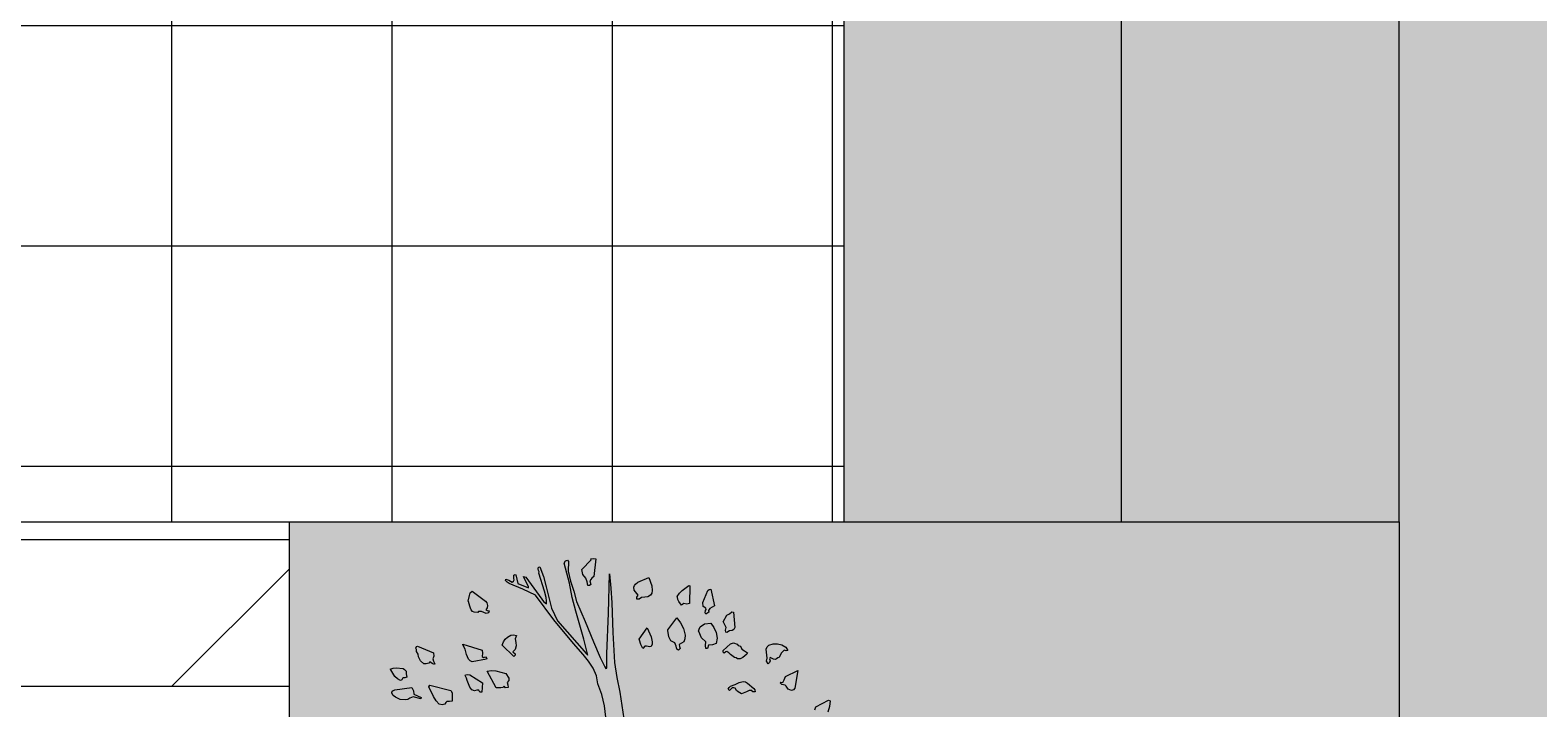
# Model space of a CAD drawing. Units: inches. Extents: x 84 to 1044, y -280 to 906.
# Tile 63 of 105: x 375 to 440, y 761 to 790. Entities that reach past the tile are written whole.
import ezdxf

# ---------------------------------------------------------------- set-up
doc = ezdxf.new("R2010")
doc.units = ezdxf.units.IN
for name, color, linetype, lineweight in [('A-ANNO-DIMS', 2, 'Continuous', 18), ('A-STAIRCASE', 144, 'Continuous', 18), ('L-HRDS', 32, 'Continuous', 18), ('L-PLNT', 114, 'Continuous', 15)]:
    doc.layers.add(name, color=color, linetype=linetype, lineweight=lineweight)
for name, color, linetype, lineweight, true_color in [('A-FLOR-PATT', 251, 'Continuous', 9, 0x705861), ('A-FLOR-STRS-PATT', 35, 'Continuous', 9, 0x947764), ('L-PLNT-PATT', 9, 'Continuous', 9, 0xafd9aa)]:
    doc.layers.add(name, color=color, linetype=linetype, lineweight=lineweight, true_color=true_color)
doc.styles.get("Standard").update_dxf_attribs({"font": 'arial.ttf'})
doc.dimstyles.get("Standard").update_dxf_attribs({"dimtxt": 0.18, "dimasz": 0.18, "dimexe": 0.18, "dimexo": 0.0625, "dimgap": 0.09, "dimtad": 0, "dimtih": 1, "dimtoh": 1, "dimdec": 4, "dimzin": 0, "dimdsep": 46, "dimtxsty": 'Standard', "dimcen": 0.09, "dimadec": 0, "dimazin": 0, "dimtfac": 1, "dimtdec": 4, "dimtofl": 0, "dimtmove": 0, "dimatfit": 3, "dimfxl": 1, "dimtolj": 1, "dimtzin": 0, "dimarcsym": 0})

# ---------------------------------------------------------------- blocks, each defined once
blk = doc.blocks.new('A$C37E508DF')
for p, q in [((0.6329, 1.5111), (0.6367, 1.5175)), ((0.6475, 1.4545), (0.6329, 1.5111)), ((0.6367, 1.5175), (0.6423, 1.5201)), ((0.6423, 1.5201), (0.6453, 1.5158)), ((0.6453, 1.5158), (0.644, 1.4879)), ((0.6826, 1.493), (0.7096, 1.5209)), ((0.7083, 1.5239), (0.7152, 1.5244)), ((0.7096, 1.5209), (0.7083, 1.5239)), ((0.7152, 1.5244), (0.7225, 1.5231)), ((0.7225, 1.5231), (0.7174, 1.4729)), ((0.4657, 1.4622), (0.4669, 1.4652)), ((0.4708, 1.4566), (0.4657, 1.4622)), ((0.4669, 1.4652), (0.4755, 1.463)), ((0.4755, 1.463), (0.4845, 1.4575)), ((0.4845, 1.4575), (0.4884, 1.4596)), ((0.4884, 1.4596), (0.4905, 1.4635)), ((0.4897, 1.4772), (0.4935, 1.4789)), ((0.4897, 1.4678), (0.4897, 1.4772)), ((0.4905, 1.4635), (0.4897, 1.4678)), ((0.4935, 1.4789), (0.4952, 1.478)), ((0.4952, 1.478), (0.5004, 1.4532)), ((0.5313, 1.4437), (0.5167, 1.4729)), ((0.5167, 1.4729), (0.5231, 1.4716)), ((0.5231, 1.4716), (0.5686, 1.409)), ((0.5583, 1.4948), (0.5596, 1.4995)), ((0.5596, 1.4905), (0.5583, 1.4948)), ((0.5596, 1.4995), (0.563, 1.5003)), ((0.5613, 1.4862), (0.5596, 1.4905)), ((0.5608, 1.4823), (0.5613, 1.4862)), ((0.5767, 1.4317), (0.5608, 1.4823)), ((0.563, 1.5003), (0.5737, 1.4733)), ((0.5737, 1.4733), (0.5814, 1.4437)), ((0.644, 1.4879), (0.6505, 1.46)), ((0.6505, 1.46), (0.6603, 1.4317)), ((0.6852, 1.4785), (0.6826, 1.493)), ((0.6946, 1.4682), (0.6852, 1.4785)), ((0.6976, 1.4579), (0.6946, 1.4682)), ((0.7109, 1.4682), (0.7053, 1.4609)), ((0.7053, 1.4609), (0.7083, 1.4502)), ((0.7174, 1.4729), (0.7109, 1.4682)), ((0.7589, 1.3691), (0.7615, 1.481)), ((0.7615, 1.481), (0.7658, 1.4395)), ((0.8421, 1.4575), (0.8739, 1.4703)), ((0.8739, 1.4703), (0.882, 1.4463)), ((0.3598, 1.403), (0.3628, 1.4189)), ((0.3628, 1.4189), (0.3649, 1.4266)), ((0.3649, 1.4266), (0.3709, 1.4317)), ((0.3709, 1.4317), (0.4086, 1.403)), ((0.4764, 1.4532), (0.4708, 1.4566)), ((0.5154, 1.4373), (0.4764, 1.4532)), ((0.5004, 1.4532), (0.5308, 1.4412)), ((0.551, 1.4197), (0.5154, 1.4373)), ((0.5308, 1.4412), (0.5313, 1.4437)), ((0.6029, 1.3494), (0.551, 1.4197)), ((0.5814, 1.4133), (0.5767, 1.4317)), ((0.5814, 1.4437), (0.5969, 1.3833)), ((0.6552, 1.4137), (0.6475, 1.4545)), ((0.6603, 1.4317), (0.668, 1.4021)), ((0.7002, 1.4476), (0.6976, 1.4579)), ((0.7049, 1.448), (0.7002, 1.4476)), ((0.7083, 1.4502), (0.7049, 1.448)), ((0.7658, 1.4395), (0.7684, 1.3979)), ((0.831, 1.4424), (0.8323, 1.4476)), ((0.8318, 1.4343), (0.831, 1.4424)), ((0.8353, 1.4292), (0.8318, 1.4343)), ((0.8323, 1.4476), (0.8357, 1.451)), ((0.8434, 1.4197), (0.8353, 1.4292)), ((0.8357, 1.451), (0.8421, 1.4575)), ((0.8391, 1.4141), (0.8434, 1.4197)), ((0.8781, 1.4197), (0.8709, 1.4154)), ((0.8816, 1.4262), (0.8781, 1.4197)), ((0.8829, 1.433), (0.8816, 1.4262)), ((0.882, 1.4463), (0.8829, 1.433)), ((0.9545, 1.4159), (0.9605, 1.4257)), ((0.9549, 1.4146), (0.9545, 1.4159)), ((0.9605, 1.4257), (0.9686, 1.4334)), ((0.9686, 1.4334), (0.9875, 1.4476)), ((0.9875, 1.4476), (0.9905, 1.4467)), ((0.9905, 1.4467), (0.9896, 1.3966)), ((1.0269, 1.3996), (1.0411, 1.433)), ((1.0411, 1.433), (1.045, 1.4365)), ((1.045, 1.4365), (1.0497, 1.4369)), ((1.0497, 1.4369), (1.0604, 1.3901)), ((0.3602, 1.4021), (0.3598, 1.403)), ((0.364, 1.3888), (0.3602, 1.4021)), ((0.3657, 1.3828), (0.364, 1.3888)), ((0.3683, 1.3781), (0.3657, 1.3828)), ((0.3718, 1.3738), (0.3683, 1.3781)), ((0.3765, 1.3713), (0.3718, 1.3738)), ((0.3885, 1.3738), (0.3872, 1.3708)), ((0.3971, 1.3734), (0.3885, 1.3738)), ((0.4039, 1.3704), (0.3971, 1.3734)), ((0.4086, 1.403), (0.4125, 1.3979)), ((0.4134, 1.3837), (0.4099, 1.3781)), ((0.4099, 1.3781), (0.4134, 1.376)), ((0.4125, 1.3979), (0.4142, 1.391)), ((0.4142, 1.391), (0.4134, 1.3837)), ((0.4134, 1.376), (0.4189, 1.3751)), ((0.4189, 1.3751), (0.4176, 1.37)), ((0.5686, 1.409), (0.5741, 1.4021)), ((0.5741, 1.4021), (0.5823, 1.3953)), ((0.5827, 1.4043), (0.5814, 1.4133)), ((0.5823, 1.3953), (0.5827, 1.4043)), ((0.5969, 1.3833), (0.6132, 1.3472)), ((0.6655, 1.3743), (0.6552, 1.4137)), ((0.6882, 1.2949), (0.6655, 1.3743)), ((0.668, 1.4021), (0.6925, 1.3455)), ((0.7684, 1.3979), (0.771, 1.3134)), ((0.8395, 1.4086), (0.8391, 1.4141)), ((0.846, 1.4086), (0.8395, 1.4086)), ((0.8528, 1.4137), (0.846, 1.4086)), ((0.8619, 1.4146), (0.8528, 1.4137)), ((0.8709, 1.4154), (0.8619, 1.4146)), ((0.9558, 1.4077), (0.9549, 1.4146)), ((0.9592, 1.4017), (0.9558, 1.4077)), ((0.966, 1.3914), (0.9592, 1.4017)), ((0.9703, 1.3944), (0.966, 1.3914)), ((0.9733, 1.3966), (0.9703, 1.3944)), ((0.9819, 1.3944), (0.9733, 1.3966)), ((0.9896, 1.3966), (0.9819, 1.3944)), ((1.0282, 1.3876), (1.0269, 1.3996)), ((1.0359, 1.3833), (1.0282, 1.3876)), ((1.0334, 1.37), (1.0351, 1.376)), ((1.0351, 1.376), (1.0368, 1.3794)), ((1.0368, 1.3794), (1.0359, 1.3833)), ((1.0471, 1.3824), (1.0432, 1.3764)), ((1.0432, 1.3764), (1.0441, 1.3717)), ((1.0604, 1.3901), (1.0471, 1.3824)), ((1.1033, 1.367), (1.1097, 1.373)), ((1.1097, 1.373), (1.114, 1.3717)), ((0.3872, 1.3708), (0.3765, 1.3713)), ((0.4108, 1.3683), (0.4039, 1.3704)), ((0.4176, 1.37), (0.4108, 1.3683)), ((0.6595, 1.2829), (0.6029, 1.3494)), ((0.6132, 1.3472), (0.6959, 1.2529)), ((0.6925, 1.3455), (0.7161, 1.2868)), ((0.7538, 1.2529), (0.7589, 1.3691)), ((0.9274, 1.3215), (0.9532, 1.3554)), ((0.9532, 1.3554), (0.9635, 1.3413)), ((0.9635, 1.3413), (0.9721, 1.325)), ((1.0197, 1.3297), (1.0321, 1.3387)), ((1.0321, 1.3387), (1.0497, 1.3404)), ((1.0359, 1.3661), (1.0334, 1.37)), ((1.0441, 1.3717), (1.0359, 1.3661)), ((1.0497, 1.3404), (1.0587, 1.3284)), ((1.0848, 1.3443), (1.0955, 1.3631)), ((1.0861, 1.343), (1.0848, 1.3443)), ((1.0938, 1.328), (1.0861, 1.343)), ((1.0955, 1.3631), (1.1033, 1.367)), ((1.114, 1.3717), (1.1183, 1.328)), ((0.4597, 1.2868), (0.4648, 1.2945)), ((0.4648, 1.2945), (0.4717, 1.3009)), ((0.4717, 1.3009), (0.4807, 1.3065)), ((0.4807, 1.3065), (0.4884, 1.3074)), ((0.4884, 1.3074), (0.4965, 1.3057)), ((0.4965, 1.3057), (0.4935, 1.2954)), ((0.4935, 1.2954), (0.4948, 1.2855)), ((0.7002, 1.2495), (0.6882, 1.2949)), ((0.771, 1.3134), (0.7761, 1.2285)), ((0.846, 1.2949), (0.8687, 1.3271)), ((0.8473, 1.2924), (0.846, 1.2949)), ((0.8507, 1.2795), (0.8473, 1.2924)), ((0.8687, 1.3271), (0.8803, 1.3014)), ((0.8803, 1.3014), (0.8833, 1.2872)), ((0.8833, 1.2872), (0.8829, 1.2808)), ((0.9279, 1.3194), (0.9274, 1.3215)), ((0.9305, 1.3018), (0.9279, 1.3194)), ((0.9365, 1.2902), (0.9305, 1.3018)), ((0.9476, 1.2842), (0.9365, 1.2902)), ((0.9721, 1.325), (0.9768, 1.3061)), ((0.9763, 1.2962), (0.9733, 1.2868)), ((0.9768, 1.3061), (0.9763, 1.2962)), ((1.0149, 1.3172), (1.0171, 1.3232)), ((1.0162, 1.3164), (1.0149, 1.3172)), ((1.0231, 1.2988), (1.0162, 1.3164)), ((1.0171, 1.3232), (1.0197, 1.3297)), ((1.0359, 1.2868), (1.0231, 1.2988)), ((1.0587, 1.3284), (1.0651, 1.3134)), ((1.0677, 1.2975), (1.0647, 1.2829)), ((1.0651, 1.3134), (1.0677, 1.2975)), ((1.0917, 1.3207), (1.0938, 1.328)), ((1.0925, 1.3151), (1.0917, 1.3207)), ((1.0955, 1.3138), (1.0925, 1.3151)), ((1.1028, 1.3185), (1.0955, 1.3138)), ((1.111, 1.3194), (1.1028, 1.3185)), ((1.1153, 1.3228), (1.111, 1.3194)), ((1.1183, 1.328), (1.1153, 1.3228)), ((0.2101, 1.2696), (0.2127, 1.2744)), ((0.2127, 1.2654), (0.2101, 1.2696)), ((0.2127, 1.2744), (0.2152, 1.2752)), ((0.2127, 1.2602), (0.2127, 1.2654)), ((0.2174, 1.2521), (0.2127, 1.2602)), ((0.2152, 1.2752), (0.2611, 1.2559)), ((0.2182, 1.2443), (0.2174, 1.2521)), ((0.2234, 1.2336), (0.2182, 1.2443)), ((0.262, 1.2465), (0.2586, 1.2388)), ((0.2611, 1.2559), (0.262, 1.2465)), ((0.3439, 1.2804), (0.3992, 1.2636)), ((0.3439, 1.2787), (0.3439, 1.2804)), ((0.3507, 1.2662), (0.3439, 1.2787)), ((0.3546, 1.2516), (0.3507, 1.2662)), ((0.3602, 1.2383), (0.3546, 1.2516)), ((0.3992, 1.2636), (0.4005, 1.2546)), ((0.4005, 1.2546), (0.3992, 1.2452)), ((0.3992, 1.2452), (0.4026, 1.2431)), ((0.4026, 1.2431), (0.4086, 1.2443)), ((0.4086, 1.2443), (0.4121, 1.2401)), ((0.4562, 1.2774), (0.4597, 1.2868)), ((0.4897, 1.2452), (0.4562, 1.2774)), ((0.4935, 1.2658), (0.4867, 1.2589)), ((0.4867, 1.2589), (0.4935, 1.2529)), ((0.4931, 1.2491), (0.4897, 1.2452)), ((0.4935, 1.2529), (0.4931, 1.2491)), ((0.4961, 1.2756), (0.4935, 1.2658)), ((0.4948, 1.2855), (0.4961, 1.2756)), ((0.6865, 1.2508), (0.6595, 1.2829)), ((0.7015, 1.2323), (0.6865, 1.2508)), ((0.6959, 1.2529), (0.7002, 1.2495)), ((0.7161, 1.2868), (0.7349, 1.2422)), ((0.7538, 1.2122), (0.7538, 1.2529)), ((0.8567, 1.2679), (0.8507, 1.2795)), ((0.8619, 1.2752), (0.8567, 1.2679)), ((0.867, 1.2752), (0.8619, 1.2752)), ((0.8713, 1.2739), (0.867, 1.2752)), ((0.8756, 1.2726), (0.8713, 1.2739)), ((0.8799, 1.2744), (0.8756, 1.2726)), ((0.8829, 1.2808), (0.8799, 1.2744)), ((0.951, 1.2748), (0.9476, 1.2842)), ((0.9532, 1.2666), (0.951, 1.2748)), ((0.9583, 1.2636), (0.9532, 1.2666)), ((0.9626, 1.2679), (0.9583, 1.2636)), ((0.9733, 1.2868), (0.9596, 1.2799)), ((0.9596, 1.2799), (0.9605, 1.2744)), ((0.9605, 1.2744), (0.9626, 1.2679)), ((1.0347, 1.2769), (1.0359, 1.2868)), ((1.0359, 1.2679), (1.0347, 1.2769)), ((1.0402, 1.2679), (1.0359, 1.2679)), ((1.0432, 1.2774), (1.0402, 1.2679)), ((1.0544, 1.2791), (1.0432, 1.2774)), ((1.0647, 1.2829), (1.0544, 1.2791)), ((1.0848, 1.2628), (1.1054, 1.2817)), ((1.0852, 1.2576), (1.0848, 1.2628)), ((1.0883, 1.2546), (1.0852, 1.2576)), ((1.0921, 1.2585), (1.0883, 1.2546)), ((1.0955, 1.2602), (1.0921, 1.2585)), ((1.1015, 1.2559), (1.0955, 1.2602)), ((1.1063, 1.2508), (1.1015, 1.2559)), ((1.1054, 1.2817), (1.1148, 1.2842)), ((1.117, 1.2422), (1.1063, 1.2508)), ((1.1148, 1.2842), (1.1247, 1.2804)), ((1.1247, 1.2804), (1.1281, 1.2765)), ((1.1281, 1.2765), (1.1341, 1.2752)), ((1.1341, 1.2752), (1.1384, 1.2666)), ((1.1384, 1.2666), (1.1461, 1.2619)), ((1.1526, 1.2521), (1.141, 1.2422)), ((1.1461, 1.2619), (1.1539, 1.2559)), ((1.1539, 1.2559), (1.1526, 1.2521)), ((1.2075, 1.2666), (1.21, 1.2726)), ((1.2096, 1.2491), (1.2075, 1.2666)), ((1.21, 1.2409), (1.2096, 1.2491)), ((1.21, 1.2726), (1.2147, 1.2774)), ((1.2147, 1.2774), (1.2276, 1.2817)), ((1.2276, 1.2817), (1.2392, 1.2817)), ((1.2392, 1.2817), (1.2521, 1.2787)), ((1.2503, 1.2551), (1.2448, 1.2431)), ((1.2585, 1.2636), (1.2503, 1.2551)), ((1.2521, 1.2787), (1.2632, 1.2722)), ((1.2645, 1.2615), (1.2585, 1.2636)), ((1.2632, 1.2722), (1.2692, 1.2628)), ((1.2692, 1.2628), (1.2645, 1.2615)), ((0.1376, 1.2092), (0.1458, 1.2126)), ((0.1389, 1.2079), (0.1376, 1.2092)), ((0.1505, 1.189), (0.1389, 1.2079)), ((0.1458, 1.2126), (0.1548, 1.2135)), ((0.1548, 1.2135), (0.1741, 1.2109)), ((0.1741, 1.2109), (0.1784, 1.2083)), ((0.1784, 1.2083), (0.1831, 1.204)), ((0.1831, 1.204), (0.1831, 1.1959)), ((0.2328, 1.2251), (0.2234, 1.2336)), ((0.2401, 1.2251), (0.2328, 1.2251)), ((0.2474, 1.2268), (0.2401, 1.2251)), ((0.2504, 1.2306), (0.2474, 1.2268)), ((0.2568, 1.2255), (0.2504, 1.2306)), ((0.2633, 1.2229), (0.2568, 1.2255)), ((0.2586, 1.2388), (0.2611, 1.2319)), ((0.2611, 1.2319), (0.265, 1.2251)), ((0.265, 1.2251), (0.2633, 1.2229)), ((0.3649, 1.2336), (0.3602, 1.2383)), ((0.3709, 1.2306), (0.3649, 1.2336)), ((0.4112, 1.2375), (0.3709, 1.2306)), ((0.4121, 1.2401), (0.4112, 1.2375)), ((0.4134, 1.204), (0.4258, 1.2058)), ((0.4391, 1.156), (0.4134, 1.204)), ((0.4258, 1.2058), (0.4382, 1.2045)), ((0.4382, 1.2045), (0.4669, 1.1972)), ((0.7148, 1.2126), (0.7015, 1.2323)), ((0.7246, 1.1908), (0.7148, 1.2126)), ((0.7349, 1.2422), (0.7482, 1.216)), ((0.7482, 1.216), (0.7508, 1.2109)), ((0.7508, 1.2109), (0.7538, 1.2122)), ((0.7761, 1.2285), (0.7821, 1.1856)), ((1.1221, 1.2418), (1.117, 1.2422)), ((1.126, 1.2388), (1.1221, 1.2418)), ((1.1337, 1.2388), (1.126, 1.2388)), ((1.141, 1.2422), (1.1337, 1.2388)), ((1.2079, 1.2323), (1.21, 1.2409)), ((1.2126, 1.2251), (1.2079, 1.2323)), ((1.2169, 1.2285), (1.2126, 1.2251)), ((1.2186, 1.2332), (1.2169, 1.2285)), ((1.2186, 1.2431), (1.2173, 1.2392)), ((1.2173, 1.2392), (1.2186, 1.2332)), ((1.2285, 1.2383), (1.2186, 1.2431)), ((1.2328, 1.2366), (1.2285, 1.2383)), ((1.2371, 1.2388), (1.2328, 1.2366)), ((1.2405, 1.2418), (1.2371, 1.2388)), ((1.2448, 1.2431), (1.2405, 1.2418)), ((1.2628, 1.1882), (1.2975, 1.2053)), ((1.2975, 1.2053), (1.2885, 1.1556)), ((0.1582, 1.1822), (0.1505, 1.189)), ((0.1668, 1.1775), (0.1582, 1.1822)), ((0.1711, 1.1792), (0.1668, 1.1775)), ((0.1728, 1.1826), (0.1711, 1.1792)), ((0.1758, 1.1847), (0.1728, 1.1826)), ((0.1788, 1.1852), (0.1758, 1.1847)), ((0.1848, 1.1865), (0.1788, 1.1852)), ((0.1831, 1.1959), (0.1848, 1.1865)), ((0.2478, 1.1594), (0.2504, 1.1637)), ((0.2607, 1.1316), (0.2478, 1.1594)), ((0.2504, 1.1637), (0.3104, 1.1487)), ((0.3507, 1.1916), (0.352, 1.1933)), ((0.355, 1.1839), (0.3507, 1.1916)), ((0.352, 1.1933), (0.3576, 1.1942)), ((0.3563, 1.177), (0.355, 1.1839)), ((0.3645, 1.1586), (0.3563, 1.177)), ((0.3576, 1.1942), (0.364, 1.1929)), ((0.364, 1.1929), (0.4005, 1.1702)), ((0.37, 1.1509), (0.3645, 1.1586)), ((0.4005, 1.1702), (0.3979, 1.1436)), ((0.4622, 1.1607), (0.458, 1.1573)), ((0.4657, 1.156), (0.4622, 1.1607)), ((0.4669, 1.1972), (0.4747, 1.1843)), ((0.4751, 1.177), (0.47, 1.1714)), ((0.47, 1.1714), (0.4721, 1.1646)), ((0.4721, 1.1646), (0.473, 1.1573)), ((0.4747, 1.1843), (0.4751, 1.177)), ((0.7281, 1.168), (0.7246, 1.1908)), ((0.7396, 1.1371), (0.7281, 1.168)), ((0.7821, 1.1856), (0.7911, 1.1436)), ((1.102, 1.1573), (1.1063, 1.1612)), ((1.1063, 1.1612), (1.1187, 1.1655)), ((1.1187, 1.1655), (1.1307, 1.1714)), ((1.1307, 1.1714), (1.1423, 1.1744)), ((1.1423, 1.1744), (1.1483, 1.1732)), ((1.1483, 1.1732), (1.1539, 1.1693)), ((1.1539, 1.1693), (1.1727, 1.1543)), ((1.2469, 1.1702), (1.2495, 1.1723)), ((1.2478, 1.1693), (1.2469, 1.1702)), ((1.2516, 1.1659), (1.2478, 1.1693)), ((1.2495, 1.1723), (1.2546, 1.1719)), ((1.2563, 1.1646), (1.2516, 1.1659)), ((1.2546, 1.1719), (1.2589, 1.1792)), ((1.2611, 1.1637), (1.2563, 1.1646)), ((1.2589, 1.1792), (1.2628, 1.1882)), ((1.2641, 1.1612), (1.2611, 1.1637)), ((1.2701, 1.1522), (1.2641, 1.1612)), ((0.1419, 1.1436), (0.1449, 1.1474)), ((0.1419, 1.141), (0.1419, 1.1436)), ((0.1462, 1.1342), (0.1419, 1.141)), ((0.1449, 1.1474), (0.1509, 1.1504)), ((0.1522, 1.1294), (0.1462, 1.1342)), ((0.1509, 1.1504), (0.1994, 1.1573)), ((0.1655, 1.1234), (0.1522, 1.1294)), ((0.181, 1.1226), (0.1655, 1.1234)), ((0.1878, 1.1234), (0.181, 1.1226)), ((0.1938, 1.1273), (0.1878, 1.1234)), ((0.2032, 1.1303), (0.1938, 1.1273)), ((0.1994, 1.1573), (0.2041, 1.1479)), ((0.2247, 1.1251), (0.2032, 1.1303)), ((0.2041, 1.1479), (0.2045, 1.138)), ((0.2045, 1.138), (0.226, 1.129)), ((0.226, 1.129), (0.2247, 1.1251)), ((0.268, 1.1196), (0.2607, 1.1316)), ((0.277, 1.1101), (0.268, 1.1196)), ((0.2984, 1.1179), (0.2959, 1.1144)), ((0.3066, 1.1179), (0.2984, 1.1179)), ((0.3134, 1.1183), (0.3066, 1.1179)), ((0.3104, 1.1487), (0.3134, 1.1423)), ((0.3134, 1.1423), (0.3139, 1.1346)), ((0.3139, 1.1346), (0.3134, 1.1183)), ((0.3778, 1.1474), (0.37, 1.1509)), ((0.3842, 1.15), (0.3778, 1.1474)), ((0.3898, 1.15), (0.3842, 1.15)), ((0.3923, 1.1436), (0.3898, 1.15)), ((0.3979, 1.1436), (0.3923, 1.1436)), ((0.4519, 1.1564), (0.4391, 1.156)), ((0.458, 1.1573), (0.4519, 1.1564)), ((0.473, 1.1573), (0.4657, 1.156)), ((0.7469, 1.1054), (0.7396, 1.1371)), ((0.7911, 1.1436), (0.8027, 1.0677)), ((1.099, 1.153), (1.102, 1.1573)), ((1.1033, 1.1487), (1.099, 1.153)), ((1.111, 1.156), (1.1033, 1.1487)), ((1.1153, 1.1564), (1.111, 1.156)), ((1.1191, 1.1556), (1.1153, 1.1564)), ((1.1226, 1.1492), (1.1191, 1.1556)), ((1.1273, 1.1453), (1.1226, 1.1492)), ((1.1367, 1.1393), (1.1273, 1.1453)), ((1.1517, 1.1453), (1.1367, 1.1393)), ((1.1586, 1.1483), (1.1517, 1.1453)), ((1.1663, 1.1487), (1.1586, 1.1483)), ((1.1697, 1.1449), (1.1663, 1.1487)), ((1.1757, 1.1449), (1.1697, 1.1449)), ((1.1727, 1.1543), (1.1749, 1.1504)), ((1.1749, 1.1504), (1.1757, 1.1449)), ((1.2791, 1.1487), (1.2701, 1.1522)), ((1.2851, 1.1509), (1.2791, 1.1487)), ((1.2885, 1.1556), (1.2851, 1.1509)), ((1.3485, 1.102), (1.385, 1.1209)), ((1.385, 1.1209), (1.3897, 1.1196)), ((1.3897, 1.1196), (1.3875, 1.1037)), ((0.2856, 1.108), (0.277, 1.1101)), ((0.2933, 1.1101), (0.2856, 1.108)), ((0.2959, 1.1144), (0.2933, 1.1101)), ((0.7512, 1.0728), (0.7469, 1.1054)), ((1.3455, 1.0934), (1.3485, 1.102)), ((1.3875, 1.1037), (1.3828, 1.087))]:
    blk.add_line(p, q)
blk = doc.blocks.new('*D62')
at = {"layer": 'A-ANNO-DIMS', "color": 0, "lineweight": -2, "transparency": 16777216}
for p, q in [((203.179, 709.183), (203.179, 905.9)), ((203.359, 905.72), (549.232, 905.72)), ((895.894, 905.72), (550.021, 905.72)), ((896.074, 400.183), (896.074, 905.9))]:
    blk.add_line(p, q, dxfattribs=at)
at = {"layer": 'A-ANNO-DIMS', "color": 0, "transparency": 16777216}
for points in [[(203.359, 905.75), (203.359, 905.69), (203.179, 905.72)], [(895.894, 905.75), (895.894, 905.69), (896.074, 905.72)]]:
    blk.add_solid(points, dxfattribs=at)
at = {"layer": 'Defpoints', "color": 0, "transparency": 16777216}
for p in [(896.074, 905.72), (203.179, 709.12), (896.074, 400.12)]:
    blk.add_point(p, dxfattribs=at)
at = {"layer": 'A-ANNO-DIMS', "color": 0, "transparency": 16777216, "insert": (549.627, 905.72), "char_height": 0.18, "attachment_point": 5}
blk.add_mtext('\\A1;692.9', dxfattribs=at)

msp = doc.modelspace()

# ---------------------------------------------------------------- hatches: boundary and pattern name
at = {"layer": 'A-FLOR-PATT', "transparency": 33554597}
h = msp.add_hatch(dxfattribs=at)
h.set_pattern_fill('ANSI37', color=256, scale=3, angle=45)
h.paths.add_polyline_path([(410.074, 847.12), (143.179, 847.12), (143.179, 769.12), (203.179, 769.12), (410.074, 769.12)])
h.paths.add_polyline_path([(254.313, 826.374, -0.414214), (254.257, 823.878, -0.414214), (251.76, 823.934), (244.439, 831.592, 0.3775), (230.555, 830.526, 0.076599), (228.51, 828.052, -0.127919), (230.803, 827.709, -0.121523), (233.469, 828.328, -0.425989), (233.291, 814.163, -0.165541), (230.889, 815.094, -0.016888), (230.578, 814.914), (236.189, 809.046, -0.414214), (236.133, 806.549, -0.414214), (233.636, 806.605, 0.414214), (238.63, 806.493), (246.415, 813.937), (254.201, 821.381, 0.414214)], flags=16)
h.paths.add_polyline_path([(241.241, 801.211), (258.998, 817.357), (267.168, 808.372), (249.545, 792.347)], flags=16)
h.paths.add_polyline_path([(262.121, 832.717, -1), (274.121, 832.717, -1)], flags=16)
h.paths.add_polyline_path([(315.269, 832.717, -1), (327.269, 832.717, -1)], flags=16)
h.paths.add_polyline_path([(322.221, 808.372), (330.392, 817.357), (348.148, 801.211), (339.844, 792.347)], flags=16)
h.paths.add_polyline_path([(344.951, 831.592, -0.372719), (358.711, 830.652), (358.966, 830.408, -0.072384), (360.879, 828.052, -0.103042), (362.667, 827.476, -0.02342), (363.022, 827.039, 0.134832), (360.058, 831.805, 0.419104)], flags=0)
h.paths.add_polyline_path([(355.753, 806.605, -0.414214), (353.257, 806.549, -0.414214), (353.201, 809.046), (358.811, 814.914, 0.234158), (363.536, 814.769, 0.403722), (362.499, 834.358, 0.41788), (342.398, 834.032), (335.076, 826.374, 0.414214), (335.188, 821.381), (342.974, 813.937), (350.76, 806.493, 0.414214)], flags=16)
h = msp.add_hatch(dxfattribs=at)
h.set_pattern_fill('DOLMIT', color=256)
h.paths.add_polyline_path([(896.074, 709.12), (833.074, 709.12), (833.074, 646.12), (833.074, 574.12), (833.074, 511.12), (896.074, 511.12)])
h.paths.add_polyline_path([(386.074, 769.12), (203.179, 769.12), (203.179, 709.12), (287.127, 709.12), (359.127, 709.12), (386.074, 709.12)])
at = {"layer": 'A-FLOR-STRS-PATT', "transparency": 33554567}
h = msp.add_hatch(color=256, dxfattribs=at)
h.dxf.hatch_style = 1
h.paths.add_polyline_path([(650.074, 91.12), (638.074, 91.12), (638.074, 67.12), (455.074, 67.12), (455.074, 55.12), (650.074, 55.12)], flags=17)
h.paths.add_polyline_path([(662.074, 91.12), (650.074, 91.12), (650.074, 55.12), (455.074, 55.12), (455.074, 43.12), (662.074, 43.12)])
h.paths.add_polyline_path([(674.074, 91.12), (671.074, 91.12), (662.074, 91.12), (662.074, 43.12), (455.074, 43.12), (455.074, 31.12), (674.074, 31.12)])
h.paths.add_polyline_path([(227.179, 151.12), (203.179, 151.12), (143.179, 151.12), (143.179, 139.12), (227.179, 139.12)])
h.paths.add_polyline_path([(227.179, 139.12), (143.179, 139.12), (143.179, 127.12), (227.179, 127.12)])
h.paths.add_polyline_path([(203.179, 271.12), (143.179, 271.12), (143.179, 259.12), (203.179, 259.12)])
h.paths.add_polyline_path([(203.179, 259.12), (143.179, 259.12), (143.179, 247.12), (203.179, 247.12)])
h.paths.add_polyline_path([(203.179, 769.12), (143.179, 769.12), (143.179, 757.12), (203.179, 757.12)])
h.paths.add_polyline_path([(203.179, 757.12), (143.179, 757.12), (143.179, 745.12), (203.179, 745.12)])
h.paths.add_polyline_path([(434.074, 847.12), (422.074, 847.12), (422.074, 769.12), (434.074, 769.12)])
h.paths.add_polyline_path([(422.074, 847.12), (410.074, 847.12), (410.074, 769.12), (422.074, 769.12)])
at = {"layer": 'L-PLNT-PATT', "transparency": 33554597}
h = msp.add_hatch(color=256, dxfattribs=at)
h.dxf.hatch_style = 1
h.paths.add_polyline_path([(434.074, 769.12), (386.074, 769.12), (386.074, 709.12), (434.074, 709.12)])
h.paths.add_polyline_path([(896.074, 847.12), (434.074, 847.12), (434.074, 769.12), (434.074, 709.12), (470.074, 709.12), (506.074, 709.12), (572.074, 709.12), (608.074, 709.12), (698.074, 709.12), (770.074, 709.12), (833.074, 709.12), (896.074, 709.12)])
h.paths.add_polyline_path([(983.074, 847.12), (896.074, 847.12), (896.074, 709.12), (896.074, 547.12), (932.074, 547.12), (983.074, 547.12)])
h.paths.add_polyline_path([(983.074, 547.12), (932.074, 547.12), (932.074, 265.12), (983.074, 265.12)])
h.paths.add_polyline_path([(203.179, 646.12), (203.179, 709.12), (203.179, 745.12), (143.179, 745.12), (143.179, 271.12), (203.179, 271.12), (203.179, 274.12), (203.179, 310.12), (203.179, 574.12)])

# ---------------------------------------------------------------- linework, layer by layer
at = {"layer": 'A-STAIRCASE'}
for p, q in [((410.074, 769.12), (410.074, 847.12)), ((422.074, 769.12), (422.074, 847.12)), ((434.074, 769.12), (434.074, 847.12))]:
    msp.add_line(p, q, dxfattribs=at)
at = {"layer": 'L-HRDS'}
for p, q in [((203.179, 769.12), (434.074, 769.12)), ((386.074, 769.12), (386.074, 709.12)), ((434.074, 769.12), (434.074, 709.12))]:
    msp.add_line(p, q, dxfattribs=at)

# ---------------------------------------------------------------- block references
at = {"layer": 'L-PLNT', "xscale": 15.19586232982809, "yscale": 15.19586232982809, "zscale": 15.19586232982809}
msp.add_blockref('A$C37E508DF', (388.36, 744.368), dxfattribs=at)

# ---------------------------------------------------------------- dimensions: what is measured, and where the dimension line sits
at = {"layer": 'A-ANNO-DIMS'}
dim = msp.add_linear_dim(base=(896.074, 905.72), p1=(203.179, 709.12), p2=(896.074, 400.12), dimstyle='Standard', override={"dimdec": 1, "dimlfac": 1, "dimrnd": 0, "dimzin": 0, "dimdsep": 46, "dimlunit": 2}, dxfattribs=at)
dim.commit()
dim.dimension.update_dxf_attribs({"geometry": '*D62', "text_midpoint": (549.627, 905.72)})

doc.saveas('drawing.dxf')
